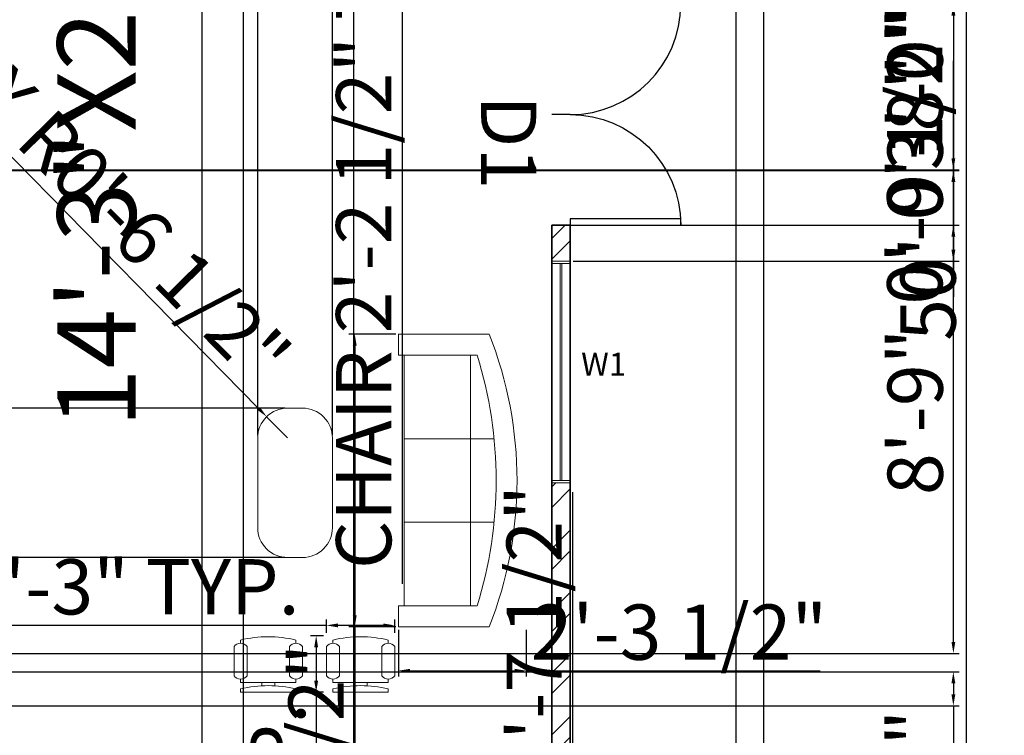
# Model space of a CAD drawing. Units: inches. Extents: x 2242 to 2870, y 1782 to 2635.
# Tile 5 of 7: x 2594 to 2807, y 2143 to 2299. Entities that reach past the tile are written whole.
import ezdxf

# ---------------------------------------------------------------- set-up
doc = ezdxf.new("R2010")
doc.units = ezdxf.units.IN
for name, color, linetype, lineweight in [('A-ANNO-DIMS', 7, 'Continuous', 18), ('A-ANNO-TEXT', 1, 'Continuous', 18), ('A-AREA-IDEN', 1, 'Continuous', 25), ('A-WALL-PATT', 253, 'Continuous', 13), ('C-PROP', 7, 'Continuous', 30), ('doors', 5, 'Continuous', 25), ('furniture', 9, 'Continuous', 18), ('walls', 7, 'Continuous', 35), ('windows', 72, 'Continuous', 18)]:
    doc.layers.add(name, color=color, linetype=linetype, lineweight=lineweight)
doc.styles.get("Standard").update_dxf_attribs({"font": 'arial.ttf'})
doc.dimstyles.new('ISO-25', dxfattribs={"dimtxt": 12, "dimasz": 2.5, "dimexe": 1.25, "dimexo": 0.625, "dimtad": 1, "dimlunit": 4, "dimtxsty": 'Standard', "dimcen": 2.5, "dimadec": 0, "dimazin": 0, "dimtfac": 1, "dimtmove": 0, "dimatfit": 3, "dimfxl": 1, "dimarcsym": 0})

# ---------------------------------------------------------------- blocks, each defined once
blk = doc.blocks.new('*U2')
for p, q in [((0, 0), (0, -5)), ((30, 0), (30, -5))]:
    blk.add_line(p, q)
blk.add_lwpolyline([(0, 0), (0, 30), (1.75, 30), (1.75, 0)], close=True)
blk.add_arc((0, 0), 30, 0, 90)
blk = doc.blocks.new('Sofa - Roundback 7 ft.')
for p, q in [((-12.00002, -32.4421), (-12.00003, -6.5971)), ((11.99997, -32.4421), (11.99998, -6.5971)), ((-36.000027, -34), (-36.000027, -11.4696)), ((-35.999844, -13.3819), (35.9998, -13.3819)), ((35.99998, -34), (35.99998, -11.4696)), ((-36.000027, -32.4421), (35.99998, -32.4421))]:
    blk.add_line(p, q)
for points in [[(-36.000027, -34), (-42.000027, -34), (-42.000027, -8)], [(41.99998, -8), (41.99998, -34), (35.99998, -34)]]:
    blk.add_lwpolyline(points)
for centre, radius, start, end in [((0, -114.25), 114.25, 68.43141, 111.5686), ((-0.00001, -127.1968), 121.1968, 72.72033, 107.2797)]:
    blk.add_arc(centre, radius, start, end)
blk = doc.blocks.new('Chair - Desk')
for p, q in [((-8.5, 0), (-8.5, -1)), ((-8.5, 0), (8.5, 0)), ((8.5, 0), (8.5, -1)), ((-8.5, -3), (-8.5, -4)), ((-8.5, -3), (8.5, -3)), ((-2, -3), (-2, -1.9355)), ((2, -1.9576), (2, -3)), ((8.5, -3), (8.5, -4)), ((-10.5, -5), (-10.5, -14)), ((-6.5, -14), (-6.5, -5)), ((6.5, -5), (6.5, -14)), ((10.5, -14), (10.5, -5)), ((-8.5, -15), (-8.5, -16)), ((8.5, -15), (8.5, -16))]:
    blk.add_line(p, q)
for centre, radius, start, end in [((0, 34.625), 36.625, 256.5803, 283.4197), ((-8.5, -6.5), 2.5, 36.8699, 143.1301), ((8.5, -6.5), 2.5, 36.8699, 143.1301), ((-8.5, -12.5), 2.5, 216.8699, 323.1301), ((8.5, -12.5), 2.5, 216.8699, 323.1301), ((0, 19.625), 36.625, 256.5803, 283.4197)]:
    blk.add_arc(centre, radius, start, end)
blk = doc.blocks.new('*D29')
at = {"layer": 'A-ANNO-DIMS', "color": 0, "lineweight": -2, "transparency": 16777216}
for p, q in [((2755.79, 2540.33), (2800.47, 2540.33)), ((2799.22, 2537.83), (2799.22, 1942.83)), ((2755.79, 1940.33), (2800.47, 1940.33))]:
    blk.add_line(p, q, dxfattribs=at)
at = {"layer": 'A-ANNO-DIMS', "color": 0, "transparency": 16777216}
for points in [[(2798.81, 2537.83), (2799.64, 2537.83), (2799.22, 2540.33)], [(2798.81, 1942.83), (2799.64, 1942.83), (2799.22, 1940.33)]]:
    blk.add_solid(points, dxfattribs=at)
at = {"layer": 'Defpoints', "color": 0, "transparency": 16777216}
for p in [(2755.16, 2540.33), (2755.16, 1940.33), (2799.22, 1940.33)]:
    blk.add_point(p, dxfattribs=at)
at = {"layer": 'A-ANNO-DIMS', "color": 0, "transparency": 16777216, "insert": (2792.47, 2240.33), "char_height": 12, "attachment_point": 5, "rotation": 90}
blk.add_mtext("50'", dxfattribs=at)
blk = doc.blocks.new('WIN-W1-48IN')
for p, q in [((0, 4), (48.12, 4)), ((0, 0), (0, 4)), ((0.5, 0), (0.5, 4)), ((0.5, 2.2), (47.62, 2.2)), ((47.62, 4), (47.62, 0)), ((48.12, 4), (48.12, 0)), ((48.12, 0), (0, 0)), ((0.5, 1.8), (47.62, 1.8))]:
    blk.add_line(p, q)
blk = doc.blocks.new('*D43')
at = {"layer": 'A-ANNO-DIMS', "color": 0, "lineweight": -2, "transparency": 16777216}
for p, q in [((2660.19, 2167.17), (2526.62, 2167.17)), ((2660.19, 2165.56), (2660.19, 2168.42)), ((2672.55, 2167.17), (2662.69, 2167.17)), ((2675.05, 2165.56), (2675.05, 2168.42))]:
    blk.add_line(p, q, dxfattribs=at)
at = {"layer": 'A-ANNO-DIMS', "color": 0, "transparency": 16777216}
for points in [[(2662.69, 2167.59), (2662.69, 2166.75), (2660.19, 2167.17)], [(2672.55, 2167.59), (2672.55, 2166.75), (2675.05, 2167.17)]]:
    blk.add_solid(points, dxfattribs=at)
at = {"layer": 'Defpoints', "color": 0, "transparency": 16777216}
for p in [(2660.19, 2167.17), (2660.19, 2164.94), (2675.05, 2164.94)]:
    blk.add_point(p, dxfattribs=at)
at = {"layer": 'A-ANNO-DIMS', "color": 0, "transparency": 16777216, "insert": (2592.15, 2174), "char_height": 12, "attachment_point": 5}
blk.add_mtext('CHAIR 1\'-3" TYP.', dxfattribs=at)
blk = doc.blocks.new('*D44')
at = {"layer": 'A-ANNO-DIMS', "color": 0, "lineweight": -2, "transparency": 16777216}
for p, q in [((2659.56, 2164.94), (2656.71, 2164.94)), ((2657.96, 2162.44), (2657.96, 2155.17)), ((2659.56, 2152.67), (2656.71, 2152.67)), ((2657.96, 2152.67), (2657.96, 2048.94))]:
    blk.add_line(p, q, dxfattribs=at)
at = {"layer": 'A-ANNO-DIMS', "color": 0, "transparency": 16777216}
for points in [[(2657.54, 2162.44), (2658.38, 2162.44), (2657.96, 2164.94)], [(2657.54, 2155.17), (2658.38, 2155.17), (2657.96, 2152.67)]]:
    blk.add_solid(points, dxfattribs=at)
at = {"layer": 'Defpoints', "color": 0, "transparency": 16777216}
for p in [(2660.19, 2164.94), (2657.96, 2152.67), (2660.19, 2152.67)]:
    blk.add_point(p, dxfattribs=at)
at = {"layer": 'A-ANNO-DIMS', "color": 0, "transparency": 16777216, "insert": (2651.13, 2099.56), "char_height": 12, "attachment_point": 5, "rotation": 90}
blk.add_mtext('1\'-0 1/2" TYP.', dxfattribs=at)
blk = doc.blocks.new('*D45')
at = {"layer": 'A-ANNO-DIMS', "color": 0, "lineweight": -2, "transparency": 16777216}
for p, q in [((2680.01, 2364.16), (2675.42, 2364.16)), ((2676.67, 2361.66), (2676.67, 2340.27)), ((2680.01, 2337.77), (2675.42, 2337.77)), ((2676.67, 2337.77), (2676.67, 2176.23))]:
    blk.add_line(p, q, dxfattribs=at)
at = {"layer": 'A-ANNO-DIMS', "color": 0, "transparency": 16777216}
for points in [[(2676.26, 2361.66), (2677.09, 2361.66), (2676.67, 2364.16)], [(2676.26, 2340.27), (2677.09, 2340.27), (2676.67, 2337.77)]]:
    blk.add_solid(points, dxfattribs=at)
at = {"layer": 'Defpoints', "color": 0, "transparency": 16777216}
for p in [(2680.63, 2364.16), (2676.67, 2337.77), (2680.63, 2337.77)]:
    blk.add_point(p, dxfattribs=at)
at = {"layer": 'A-ANNO-DIMS', "color": 0, "transparency": 16777216, "insert": (2669.84, 2255.75), "char_height": 12, "attachment_point": 5, "rotation": 90}
blk.add_mtext('CHAIR 2\'-2 1/2" TYP.', dxfattribs=at)
blk = doc.blocks.new('*D52')
at = {"layer": 'A-ANNO-DIMS', "color": 0, "lineweight": -2, "transparency": 16777216}
for p, q in [((2713.71, 2132.29), (2713.71, 2196.1)), ((2706.57, 2132.29), (2714.96, 2132.29)), ((2713.71, 2103.53), (2713.71, 2129.79)), ((2706.57, 2101.03), (2714.96, 2101.03))]:
    blk.add_line(p, q, dxfattribs=at)
at = {"layer": 'A-ANNO-DIMS', "color": 0, "transparency": 16777216}
for points in [[(2713.29, 2129.79), (2714.12, 2129.79), (2713.71, 2132.29)], [(2713.29, 2103.53), (2714.12, 2103.53), (2713.71, 2101.03)]]:
    blk.add_solid(points, dxfattribs=at)
at = {"layer": 'Defpoints', "color": 0, "transparency": 16777216}
for p in [(2705.95, 2132.29), (2713.71, 2132.29), (2705.95, 2101.03)]:
    blk.add_point(p, dxfattribs=at)
at = {"layer": 'A-ANNO-DIMS', "color": 0, "transparency": 16777216, "insert": (2706.88, 2165.45), "char_height": 12, "attachment_point": 5, "rotation": 90}
blk.add_mtext('2\'-7 1/2"', dxfattribs=at)
blk = doc.blocks.new('*D53')
at = {"layer": 'A-ANNO-DIMS', "color": 0, "lineweight": -2, "transparency": 16777216}
for p, q in [((2675.25, 2230.42), (2665.09, 2230.42)), ((2666.34, 2227.92), (2666.34, 2169.35)), ((2675.25, 2166.85), (2665.09, 2166.85)), ((2666.34, 2166.85), (2666.34, 2053))]:
    blk.add_line(p, q, dxfattribs=at)
at = {"layer": 'A-ANNO-DIMS', "color": 0, "transparency": 16777216}
for points in [[(2665.92, 2227.92), (2666.76, 2227.92), (2666.34, 2230.42)], [(2665.92, 2169.35), (2666.76, 2169.35), (2666.34, 2166.85)]]:
    blk.add_solid(points, dxfattribs=at)
at = {"layer": 'Defpoints', "color": 0, "transparency": 16777216}
for p in [(2675.87, 2230.42), (2666.34, 2166.85), (2675.87, 2166.85)]:
    blk.add_point(p, dxfattribs=at)
at = {"layer": 'A-ANNO-DIMS', "color": 0, "transparency": 16777216, "insert": (2659.5, 2108.68), "char_height": 12, "attachment_point": 5, "rotation": 90}
blk.add_mtext('SOFA 5\'-3 1/2"', dxfattribs=at)
blk = doc.blocks.new('*D54')
at = {"layer": 'A-ANNO-DIMS', "color": 0, "lineweight": -2, "transparency": 16777216}
for p, q in [((2675.87, 2166.23), (2675.87, 2156.07)), ((2703.62, 2166.23), (2703.62, 2156.07)), ((2678.37, 2157.32), (2701.12, 2157.32)), ((2703.62, 2157.32), (2767.44, 2157.32))]:
    blk.add_line(p, q, dxfattribs=at)
at = {"layer": 'A-ANNO-DIMS', "color": 0, "transparency": 16777216}
for points in [[(2678.37, 2157.74), (2678.37, 2156.9), (2675.87, 2157.32)], [(2701.12, 2157.74), (2701.12, 2156.9), (2703.62, 2157.32)]]:
    blk.add_solid(points, dxfattribs=at)
at = {"layer": 'Defpoints', "color": 0, "transparency": 16777216}
for p in [(2675.87, 2166.85), (2703.62, 2166.85), (2703.62, 2157.32)]:
    blk.add_point(p, dxfattribs=at)
at = {"layer": 'A-ANNO-DIMS', "color": 0, "transparency": 16777216, "insert": (2736.78, 2164.15), "char_height": 12, "attachment_point": 5}
blk.add_mtext('2\'-3 1/2"', dxfattribs=at)
blk = doc.blocks.new('*D62')
at = {"layer": 'A-ANNO-DIMS', "color": 0, "lineweight": -2, "transparency": 16777216}
for p, q in [((2537.37, 2302.1), (2797.66, 2302.1)), ((2796.41, 2299.6), (2796.41, 2268.6)), ((2537.37, 2266.1), (2797.66, 2266.1))]:
    blk.add_line(p, q, dxfattribs=at)
at = {"layer": 'A-ANNO-DIMS', "color": 0, "transparency": 16777216}
for points in [[(2796, 2299.6), (2796.83, 2299.6), (2796.41, 2302.1)], [(2796, 2268.6), (2796.83, 2268.6), (2796.41, 2266.1)]]:
    blk.add_solid(points, dxfattribs=at)
at = {"layer": 'Defpoints', "color": 0, "transparency": 16777216}
for p in [(2536.74, 2302.1), (2536.74, 2266.1), (2796.41, 2266.1)]:
    blk.add_point(p, dxfattribs=at)
at = {"layer": 'A-ANNO-DIMS', "color": 0, "transparency": 16777216, "insert": (2789.66, 2284.1), "char_height": 12, "attachment_point": 5, "rotation": 90}
blk.add_mtext('3\'-0"', dxfattribs=at)
blk = doc.blocks.new('*D64')
at = {"layer": 'A-ANNO-DIMS', "color": 0, "lineweight": -2, "transparency": 16777216}
for p, q in [((2642.16, 2049.72), (2642.16, 2611.83)), ((2644.66, 2610.58), (2663.66, 2610.58)), ((2666.16, 2049.72), (2666.16, 2611.83)), ((2666.16, 2610.58), (2702.02, 2610.58))]:
    blk.add_line(p, q, dxfattribs=at)
at = {"layer": 'A-ANNO-DIMS', "color": 0, "transparency": 16777216}
for points in [[(2644.66, 2611), (2644.66, 2610.17), (2642.16, 2610.58)], [(2663.66, 2611), (2663.66, 2610.17), (2666.16, 2610.58)]]:
    blk.add_solid(points, dxfattribs=at)
at = {"layer": 'Defpoints', "color": 0, "transparency": 16777216}
for p in [(2666.16, 2610.58), (2642.16, 2049.1), (2666.16, 2049.1)]:
    blk.add_point(p, dxfattribs=at)
at = {"layer": 'A-ANNO-DIMS', "color": 0, "transparency": 16777216, "insert": (2685.34, 2617.34), "char_height": 12, "attachment_point": 5}
blk.add_mtext('2\'-0"', dxfattribs=at)
blk = doc.blocks.new('*D66')
at = {"layer": 'A-ANNO-DIMS', "color": 0, "lineweight": -2, "transparency": 16777216}
for p, q in [((2713.79, 2311.76), (2797.66, 2311.76)), ((2796.41, 2309.26), (2796.41, 2304.6)), ((2713.79, 2302.1), (2797.66, 2302.1)), ((2796.41, 2302.1), (2796.41, 2238.49))]:
    blk.add_line(p, q, dxfattribs=at)
at = {"layer": 'A-ANNO-DIMS', "color": 0, "transparency": 16777216}
for points in [[(2796, 2309.26), (2796.83, 2309.26), (2796.41, 2311.76)], [(2796, 2304.6), (2796.83, 2304.6), (2796.41, 2302.1)]]:
    blk.add_solid(points, dxfattribs=at)
at = {"layer": 'Defpoints', "color": 0, "transparency": 16777216}
for p in [(2713.16, 2311.76), (2713.16, 2302.1), (2796.41, 2302.1)]:
    blk.add_point(p, dxfattribs=at)
at = {"layer": 'A-ANNO-DIMS', "color": 0, "transparency": 16777216, "insert": (2789.58, 2269.04), "char_height": 12, "attachment_point": 5, "rotation": 90}
blk.add_mtext('0\'-9 1/2"', dxfattribs=at)
blk = doc.blocks.new('*D67')
at = {"layer": 'A-ANNO-DIMS', "color": 0, "lineweight": -2, "transparency": 16777216}
for p, q in [((2796.41, 2254.1), (2796.41, 2289.75)), ((2713.79, 2254.1), (2797.66, 2254.1)), ((2796.41, 2248.75), (2796.41, 2251.6)), ((2713.79, 2246.25), (2797.66, 2246.25))]:
    blk.add_line(p, q, dxfattribs=at)
at = {"layer": 'A-ANNO-DIMS', "color": 0, "transparency": 16777216}
for points in [[(2796, 2251.6), (2796.83, 2251.6), (2796.41, 2254.1)], [(2796, 2248.75), (2796.83, 2248.75), (2796.41, 2246.25)]]:
    blk.add_solid(points, dxfattribs=at)
at = {"layer": 'Defpoints', "color": 0, "transparency": 16777216}
for p in [(2713.16, 2254.1), (2796.41, 2254.1), (2713.16, 2246.25)]:
    blk.add_point(p, dxfattribs=at)
at = {"layer": 'A-ANNO-DIMS', "color": 0, "transparency": 16777216, "insert": (2789.66, 2273.17), "char_height": 12, "attachment_point": 5, "rotation": 90}
blk.add_mtext('0\'-8"', dxfattribs=at)
blk = doc.blocks.new('*D74')
at = {"layer": 'A-ANNO-DIMS', "color": 0, "lineweight": -2, "transparency": 16777216}
for p, q in [((2645.26, 2208.5), (2645.26, 2611.83)), ((2647.76, 2610.58), (2658.99, 2610.58)), ((2661.49, 2208.5), (2661.49, 2611.83)), ((2661.49, 2610.58), (2696.01, 2610.58))]:
    blk.add_line(p, q, dxfattribs=at)
at = {"layer": 'A-ANNO-DIMS', "color": 0, "transparency": 16777216}
for points in [[(2647.76, 2611), (2647.76, 2610.17), (2645.26, 2610.58)], [(2658.99, 2611), (2658.99, 2610.17), (2661.49, 2610.58)]]:
    blk.add_solid(points, dxfattribs=at)
at = {"layer": 'Defpoints', "color": 0, "transparency": 16777216}
for p in [(2661.49, 2610.58), (2645.26, 2207.87), (2661.49, 2207.87)]:
    blk.add_point(p, dxfattribs=at)
at = {"layer": 'A-ANNO-DIMS', "color": 0, "transparency": 16777216, "insert": (2680, 2617.23), "char_height": 12, "attachment_point": 5}
blk.add_mtext('1\'-4"', dxfattribs=at)
blk = doc.blocks.new('*D75')
at = {"layer": 'A-ANNO-DIMS', "color": 0, "lineweight": -2, "transparency": 16777216}
for p, q in [((2266.89, 2214.36), (2266.89, 2278.18)), ((2651.13, 2214.36), (2265.64, 2214.36)), ((2266.89, 2184.4), (2266.89, 2211.86)), ((2651.13, 2181.9), (2265.64, 2181.9))]:
    blk.add_line(p, q, dxfattribs=at)
at = {"layer": 'A-ANNO-DIMS', "color": 0, "transparency": 16777216}
for points in [[(2266.47, 2211.86), (2267.3, 2211.86), (2266.89, 2214.36)], [(2266.47, 2184.4), (2267.3, 2184.4), (2266.89, 2181.9)]]:
    blk.add_solid(points, dxfattribs=at)
at = {"layer": 'Defpoints', "color": 0, "transparency": 16777216}
for p in [(2266.89, 2214.36), (2651.75, 2214.36), (2651.75, 2181.9)]:
    blk.add_point(p, dxfattribs=at)
at = {"layer": 'A-ANNO-DIMS', "color": 0, "transparency": 16777216, "insert": (2260.06, 2247.52), "char_height": 12, "attachment_point": 5, "rotation": 90}
blk.add_mtext('2\'-8 1/2"', dxfattribs=at)
blk = doc.blocks.new('*D77')
at = {"layer": 'A-ANNO-DIMS', "color": 0, "lineweight": -2, "transparency": 16777216}
for p, q in [((2393.37, 2157.1), (2797.66, 2157.1)), ((2796.41, 2154.6), (2796.41, 2152.19)), ((2393.37, 2149.69), (2797.66, 2149.69)), ((2796.41, 2149.69), (2796.41, 2086.08))]:
    blk.add_line(p, q, dxfattribs=at)
at = {"layer": 'A-ANNO-DIMS', "color": 0, "transparency": 16777216}
for points in [[(2796, 2154.6), (2796.83, 2154.6), (2796.41, 2157.1)], [(2796, 2152.19), (2796.83, 2152.19), (2796.41, 2149.69)]]:
    blk.add_solid(points, dxfattribs=at)
at = {"layer": 'Defpoints', "color": 0, "transparency": 16777216}
for p in [(2392.74, 2157.1), (2392.74, 2149.69), (2796.41, 2149.69)]:
    blk.add_point(p, dxfattribs=at)
at = {"layer": 'A-ANNO-DIMS', "color": 0, "transparency": 16777216, "insert": (2789.58, 2116.64), "char_height": 12, "attachment_point": 5, "rotation": 90}
blk.add_mtext('0\'-7 1/2"', dxfattribs=at)
blk = doc.blocks.new('*D80')
at = {"layer": 'A-ANNO-DIMS', "color": 0, "lineweight": -2, "transparency": 16777216}
for p, q in [((2393.37, 2265.99), (2797.66, 2265.99)), ((2796.41, 2163.6), (2796.41, 2263.49)), ((2393.37, 2161.1), (2797.66, 2161.1))]:
    blk.add_line(p, q, dxfattribs=at)
at = {"layer": 'A-ANNO-DIMS', "color": 0, "transparency": 16777216}
for points in [[(2796, 2263.49), (2796.83, 2263.49), (2796.41, 2265.99)], [(2796, 2163.6), (2796.83, 2163.6), (2796.41, 2161.1)]]:
    blk.add_solid(points, dxfattribs=at)
at = {"layer": 'Defpoints', "color": 0, "transparency": 16777216}
for p in [(2392.74, 2265.99), (2796.41, 2265.99), (2392.74, 2161.1)]:
    blk.add_point(p, dxfattribs=at)
at = {"layer": 'A-ANNO-DIMS', "color": 0, "transparency": 16777216, "insert": (2789.66, 2213.55), "char_height": 12, "attachment_point": 5, "rotation": 90}
blk.add_mtext('8\'-9"', dxfattribs=at)
blk = doc.blocks.new('*D82')
at = {"layer": 'A-ANNO-DIMS', "color": 0, "lineweight": -2, "transparency": 16777216}
for p, q in [((2633.16, 2610.58), (2597.51, 2610.58)), ((2633.16, 2049.72), (2633.16, 2611.83)), ((2639.66, 2610.58), (2635.66, 2610.58)), ((2642.16, 2049.72), (2642.16, 2611.83))]:
    blk.add_line(p, q, dxfattribs=at)
at = {"layer": 'A-ANNO-DIMS', "color": 0, "transparency": 16777216}
for points in [[(2635.66, 2611), (2635.66, 2610.17), (2633.16, 2610.58)], [(2639.66, 2611), (2639.66, 2610.17), (2642.16, 2610.58)]]:
    blk.add_solid(points, dxfattribs=at)
at = {"layer": 'Defpoints', "color": 0, "transparency": 16777216}
for p in [(2633.16, 2610.58), (2633.16, 2049.1), (2642.16, 2049.1)]:
    blk.add_point(p, dxfattribs=at)
at = {"layer": 'A-ANNO-DIMS', "color": 0, "transparency": 16777216, "insert": (2614.09, 2617.34), "char_height": 12, "attachment_point": 5}
blk.add_mtext('0\'-9"', dxfattribs=at)
blk = doc.blocks.new('*D88')
at = {"layer": 'A-ANNO-DIMS', "color": 0, "lineweight": -2, "transparency": 16777216}
for p, q in [((2574.38, 2286.56), (2645.45, 2214.28)), ((2651.75, 2207.87), (2647.2, 2212.5))]:
    blk.add_line(p, q, dxfattribs=at)
at = {"layer": 'A-ANNO-DIMS', "color": 0, "transparency": 16777216}
blk.add_solid([(2645.74, 2214.58), (2645.15, 2213.99), (2647.2, 2212.5)], dxfattribs=at)
at = {"layer": 'Defpoints', "color": 0, "transparency": 16777216}
for p in [(2647.2, 2212.5), (2651.75, 2207.87)]:
    blk.add_point(p, dxfattribs=at)
at = {"layer": 'A-ANNO-DIMS', "color": 0, "transparency": 16777216, "insert": (2613.91, 2256.1), "char_height": 12, "attachment_point": 5, "rotation": 314.5145}
blk.add_mtext('4X R0\'-6 1/2"', dxfattribs=at)

msp = doc.modelspace()

# ---------------------------------------------------------------- hatches: boundary and pattern name
at = {"layer": 'A-WALL-PATT'}
h = msp.add_hatch(dxfattribs=at)
h.set_pattern_fill('ANSI32', color=256)
h.paths.add_polyline_path([(2713.164, 2254.097), (2709.164, 2254.097), (2709.164, 2246.255), (2713.164, 2246.255)])
h = msp.add_hatch(dxfattribs=at)
h.set_pattern_fill('ANSI32', color=256)
h.paths.add_polyline_path([(2713.164, 2198.138), (2709.164, 2198.138), (2709.164, 2043.592), (2713.164, 2043.592)])

# ---------------------------------------------------------------- linework, layer by layer
at = {"layer": 'C-PROP'}
for p, q in [((2755.164, 2540.335), (2755.164, 1940.335)), ((2749.164, 2534.335), (2749.164, 1945.097))]:
    msp.add_line(p, q, dxfattribs=at)
at = {"layer": 'furniture'}
msp.add_lwpolyline([(2645.258, 2188.392, 0.4142136), (2651.751, 2181.899), (2654.998, 2181.899, 0.4142136), (2661.491, 2188.392), (2661.491, 2207.871, 0.4142136), (2654.998, 2214.364), (2651.751, 2214.364, 0.4142136), (2645.258, 2207.871)], format="xyb", close=True, dxfattribs=at)
at = {"layer": 'walls'}
for p, q in [((2713.164, 2254.097), (2709.164, 2254.097)), ((2709.164, 2254.097), (2709.164, 1961.097)), ((2713.164, 2254.097), (2713.164, 2254.097)), ((2713.164, 2254.097), (2713.164, 1957.097))]:
    msp.add_line(p, q, dxfattribs=at)

# ---------------------------------------------------------------- block references
at = {"layer": 'doors', "yscale": 0.8, "zscale": 0.8, "rotation": 270}
for p, xscale in [((2713.164, 2302.097), 0.8), ((2713.164, 2254.097), -0.8)]:
    msp.add_blockref('*U2', p, dxfattribs=dict(at, xscale=xscale))
at = {"layer": 'furniture'}
for name, p, xscale, yscale, zscale, rotation in [('Sofa - Roundback 7 ft.', (2701.603, 2198.638), 0.7567552153399788, 0.7567552153399788, 0.7567552153399788, 270), ('Chair - Desk', (2647.543, 2152.672), 0.7077236892588391, 0.7077236892588391, 0.7077236892588391, 180), ('Chair - Desk', (2667.62, 2152.672), 0.7077236892588391, 0.7077236892588391, 0.7077236892588391, 180)]:
    msp.add_blockref(name, p, dxfattribs=dict(at, xscale=xscale, yscale=yscale, zscale=zscale, rotation=rotation))
at = {"layer": 'windows', "rotation": 89.99999999999946}
msp.add_blockref('WIN-W1-48IN', (2713.164, 2198.139), dxfattribs=at)

# ---------------------------------------------------------------- texts
at = {"layer": 'A-ANNO-TEXT', "insert": (2705.791, 2282.244), "char_height": 12, "attachment_point": 1, "rotation": 270}
msp.add_mtext_dynamic_manual_height_columns('D1', width=2.16795, gutter_width=12.5, heights=[0], dxfattribs=at)
at = {"layer": 'A-ANNO-TEXT', "insert": (2715.544, 2226.388), "char_height": 5, "attachment_point": 1}
msp.add_mtext_dynamic_manual_height_columns('W1', width=1.76313, gutter_width=25, heights=[0], dxfattribs=at)
at = {"layer": 'A-AREA-IDEN', "insert": (2573.308, 2210.091), "char_height": 17.04609, "attachment_point": 1, "rotation": 90}
msp.add_mtext_dynamic_manual_height_columns('LIVINGROOM\\P14\'-3"X27\'-3"', width=6.2214, gutter_width=17.756, heights=[0], dxfattribs=at)

# ---------------------------------------------------------------- dimensions: what is measured, and where the dimension line sits
at = {"layer": 'A-ANNO-DIMS'}
for base, p1, p2, picture, middle in [((2633.164, 2610.585), (2642.164, 2049.097), (2633.164, 2049.097), '*D82', (2614.089, 2617.337)), ((2666.164, 2610.585), (2642.164, 2049.097), (2666.164, 2049.097), '*D64', (2685.34, 2617.337)), ((2661.491, 2610.585), (2645.258, 2207.871), (2661.491, 2207.871), '*D74', (2680, 2617.234)), ((2703.621, 2157.32), (2675.874, 2166.855), (2703.621, 2166.855), '*D54', (2736.779, 2164.153))]:
    dim = msp.add_linear_dim(base=base, p1=p1, p2=p2, dimstyle='ISO-25', override={"dimdec": 1, "dimlfac": 1, "dimrnd": 0, "dimzin": 1, "dimdsep": 46, "dimlunit": 4, "dimfrac": 2}, dxfattribs=at)
    dim.commit()
    dim.dimension.update_dxf_attribs({"geometry": picture, "text_midpoint": middle})
for base, p1, p2, override, picture, middle in [((2799.223, 1940.335), (2755.164, 2540.335), (2755.164, 1940.335), {"dimclrd": 0, "dimclre": 0, "dimclrt": 0}, '*D29', (2792.471, 2240.335)), ((2796.414, 2302.097), (2713.164, 2311.761), (2713.164, 2302.097), {"dimdec": 1, "dimlfac": 1, "dimrnd": 0, "dimzin": 1, "dimdsep": 46, "dimlunit": 4, "dimfrac": 2}, '*D66', (2789.584, 2269.042)), ((2796.414, 2266.097), (2536.745, 2302.097), (2536.745, 2266.097), {"dimdec": 1, "dimlfac": 1, "dimrnd": 0, "dimzin": 1, "dimdsep": 46, "dimlunit": 4, "dimfrac": 2}, '*D62', (2789.658, 2284.097)), ((2796.414, 2254.097), (2713.164, 2246.255), (2713.164, 2254.097), {"dimdec": 1, "dimlfac": 1, "dimrnd": 0, "dimzin": 1, "dimdsep": 46, "dimlunit": 4, "dimfrac": 2}, '*D67', (2789.662, 2273.172)), ((2266.887, 2214.364), (2651.751, 2181.899), (2651.751, 2214.364), {"dimdec": 1, "dimlfac": 1, "dimrnd": 0, "dimzin": 1, "dimdsep": 46, "dimlunit": 4, "dimfrac": 2}, '*D75', (2260.057, 2247.522)), ((2796.414, 2265.993), (2392.745, 2161.097), (2392.745, 2265.993), {"dimdec": 1, "dimlfac": 1, "dimrnd": 0, "dimzin": 1, "dimdsep": 46, "dimlunit": 4, "dimfrac": 2}, '*D80', (2789.662, 2213.545)), ((2713.706, 2132.289), (2705.947, 2101.027), (2705.947, 2132.289), {"dimdec": 1, "dimlfac": 1, "dimrnd": 0, "dimzin": 1, "dimdsep": 46, "dimlunit": 4, "dimfrac": 2}, '*D52', (2706.876, 2165.446)), ((2796.414, 2149.693), (2392.745, 2157.097), (2392.745, 2149.693), {"dimdec": 1, "dimlfac": 1, "dimrnd": 0, "dimzin": 1, "dimdsep": 46, "dimlunit": 4, "dimfrac": 2}, '*D77', (2789.584, 2116.638))]:
    dim = msp.add_linear_dim(base=base, p1=p1, p2=p2, angle=90, dimstyle='ISO-25', override=override, dxfattribs=at)
    dim.commit()
    dim.dimension.update_dxf_attribs({"geometry": picture, "text_midpoint": middle})
for base, p1, p2, angle, text, picture, middle in [((2676.674, 2337.767), (2680.633, 2364.159), (2680.633, 2337.767), 270, 'CHAIR <> TYP.', '*D45', (2669.845, 2255.75)), ((2666.339, 2166.855), (2675.874, 2230.422), (2675.874, 2166.855), 270, 'SOFA <>', '*D53', (2659.501, 2108.678)), ((2660.189, 2167.169), (2675.051, 2164.94), (2660.189, 2164.94), 180, 'CHAIR <> TYP.', '*D43', (2592.152, 2174.003)), ((2657.959, 2152.672), (2660.189, 2164.94), (2660.189, 2152.672), 270, '<> TYP.', '*D44', (2651.13, 2099.558))]:
    dim = msp.add_linear_dim(base=base, p1=p1, p2=p2, angle=angle, text=text, dimstyle='ISO-25', override={"dimdec": 1, "dimlfac": 1, "dimrnd": 0, "dimzin": 1, "dimdsep": 46, "dimlunit": 4, "dimfrac": 2}, dxfattribs=at)
    dim.commit()
    dim.dimension.update_dxf_attribs({"geometry": picture, "text_midpoint": middle})
dim = msp.add_radius_dim(center=(2651.751, 2207.871), mpoint=(2647.199, 2212.501), text='4X <>', dimstyle='ISO-25', override={"dimdec": 1, "dimlfac": 1, "dimrnd": 0, "dimzin": 1, "dimdsep": 46, "dimlunit": 4, "dimfrac": 2}, dxfattribs=at)
dim.commit()
dim.dimension.update_dxf_attribs({"geometry": '*D88', "text_midpoint": (2613.908, 2256.103)})

doc.saveas('drawing.dxf')
